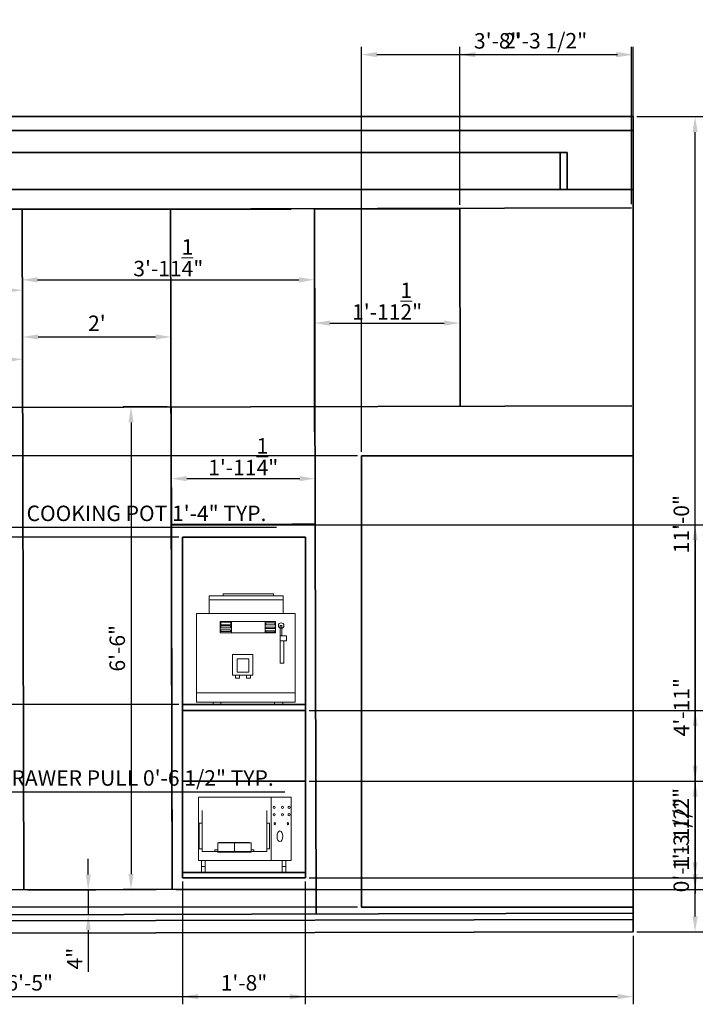
# Model space of a CAD drawing. Units: inches. Extents: x 1464 to 1689, y 996 to 1156.
# Tile 2 of 2: x 1578 to 1689, y 997 to 1156. Entities that reach past the tile are written whole.
import ezdxf

# ---------------------------------------------------------------- set-up
doc = ezdxf.new("R2010")
doc.units = ezdxf.units.IN
for name, color, linetype, lineweight in [('A-ANNO-DIMS', 2, 'Continuous', 18), ('A-ELEV', 7, 'Continuous', 35), ('A-EQPM', 9, 'Continuous', 18)]:
    doc.layers.add(name, color=color, linetype=linetype, lineweight=lineweight)
doc.styles.get("Standard").update_dxf_attribs({"font": 'arial.ttf'})
doc.dimstyles.new('ISO-25', dxfattribs={"dimtxt": 2.5, "dimasz": 2.5, "dimexe": 1.25, "dimexo": 0.625, "dimtad": 1, "dimdec": 4, "dimlunit": 4, "dimtxsty": 'Standard', "dimcen": 2.5, "dimadec": 0, "dimazin": 0, "dimtfac": 1, "dimtdec": 4, "dimtmove": 0, "dimatfit": 3, "dimfxl": 1, "dimarcsym": 0})

# ---------------------------------------------------------------- blocks, each defined once
blk = doc.blocks.new('*D3')
at = {"layer": 'A-ANNO-DIMS', "color": 0, "lineweight": -2, "transparency": 16777216}
for p, q in [((1534.7, 1124.64), (1534.7, 1110.94)), ((1578.2, 1124.64), (1578.2, 1110.94)), ((1575.7, 1112.19), (1537.2, 1112.19))]:
    blk.add_line(p, q, dxfattribs=at)
at = {"layer": 'A-ANNO-DIMS', "color": 0, "transparency": 16777216}
for points in [[(1537.2, 1112.6), (1537.2, 1111.77), (1534.7, 1112.19)], [(1575.7, 1112.6), (1575.7, 1111.77), (1578.2, 1112.19)]]:
    blk.add_solid(points, dxfattribs=at)
at = {"layer": 'Defpoints', "color": 0, "transparency": 16777216}
for p in [(1534.7, 1125.27), (1578.2, 1125.27), (1534.7, 1112.19)]:
    blk.add_point(p, dxfattribs=at)
at = {"layer": 'A-ANNO-DIMS', "color": 0, "transparency": 16777216, "insert": (1556.45, 1115.76), "char_height": 2.5, "attachment_point": 5}
blk.add_mtext('3\'-7{\\H1x;\\S1/2;}"', dxfattribs=at)
blk = doc.blocks.new('*D5')
at = {"layer": 'A-ANNO-DIMS', "color": 0, "lineweight": -2, "transparency": 16777216}
for p, q in [((1601.65, 1093.32), (1594.55, 1093.32)), ((1595.8, 1090.82), (1595.8, 1017.82)), ((1601.83, 1015.32), (1594.55, 1015.32))]:
    blk.add_line(p, q, dxfattribs=at)
at = {"layer": 'A-ANNO-DIMS', "color": 0, "transparency": 16777216}
for points in [[(1595.39, 1090.82), (1596.22, 1090.82), (1595.8, 1093.32)], [(1595.39, 1017.82), (1596.22, 1017.82), (1595.8, 1015.32)]]:
    blk.add_solid(points, dxfattribs=at)
at = {"layer": 'Defpoints', "color": 0, "transparency": 16777216}
for p in [(1602.28, 1093.32), (1595.8, 1015.32), (1602.45, 1015.32)]:
    blk.add_point(p, dxfattribs=at)
at = {"layer": 'A-ANNO-DIMS', "color": 0, "transparency": 16777216, "insert": (1593.9, 1054.32), "char_height": 2.5, "attachment_point": 5, "rotation": 90}
blk.add_mtext('6\'-6"', dxfattribs=at)
blk = doc.blocks.new('*D7')
at = {"layer": 'A-ANNO-DIMS', "color": 0, "lineweight": -2, "transparency": 16777216}
for p, q in [((1602.32, 1074.89), (1602.32, 1082.98)), ((1625.57, 1074.89), (1625.57, 1082.98)), ((1623.07, 1081.73), (1604.82, 1081.73))]:
    blk.add_line(p, q, dxfattribs=at)
at = {"layer": 'A-ANNO-DIMS', "color": 0, "transparency": 16777216}
for points in [[(1604.82, 1082.15), (1604.82, 1081.32), (1602.32, 1081.73)], [(1623.07, 1082.15), (1623.07, 1081.32), (1625.57, 1081.73)]]:
    blk.add_solid(points, dxfattribs=at)
at = {"layer": 'Defpoints', "color": 0, "transparency": 16777216}
for p in [(1602.32, 1081.73), (1602.32, 1074.27), (1625.57, 1074.27)]:
    blk.add_point(p, dxfattribs=at)
at = {"layer": 'A-ANNO-DIMS', "color": 0, "transparency": 16777216, "insert": (1613.94, 1085.28), "char_height": 2.5, "attachment_point": 5}
blk.add_mtext('1\'-11{\\H1x;\\S1/4;}"', dxfattribs=at)
blk = doc.blocks.new('*D8')
at = {"layer": 'A-ANNO-DIMS', "color": 0, "lineweight": -2, "transparency": 16777216}
for p, q in [((1625.45, 1124.75), (1625.45, 1105.63)), ((1648.95, 1124.75), (1648.95, 1105.63)), ((1627.95, 1106.88), (1646.45, 1106.88))]:
    blk.add_line(p, q, dxfattribs=at)
at = {"layer": 'A-ANNO-DIMS', "color": 0, "transparency": 16777216}
for points in [[(1627.95, 1107.29), (1627.95, 1106.46), (1625.45, 1106.88)], [(1646.45, 1107.29), (1646.45, 1106.46), (1648.95, 1106.88)]]:
    blk.add_solid(points, dxfattribs=at)
at = {"layer": 'Defpoints', "color": 0, "transparency": 16777216}
for p in [(1625.45, 1125.37), (1648.95, 1125.37), (1648.95, 1106.88)]:
    blk.add_point(p, dxfattribs=at)
at = {"layer": 'A-ANNO-DIMS', "color": 0, "transparency": 16777216, "insert": (1637.2, 1110.43), "char_height": 2.5, "attachment_point": 5}
blk.add_mtext('1\'-11{\\H1x;\\S1/2;}"', dxfattribs=at)
blk = doc.blocks.new('*D9')
at = {"layer": 'A-ANNO-DIMS', "color": 0, "lineweight": -2, "transparency": 16777216}
for p, q in [((1554.53, 1093.84), (1554.53, 1102.26)), ((1578.28, 1093.89), (1578.28, 1102.26)), ((1557.03, 1101.01), (1575.78, 1101.01))]:
    blk.add_line(p, q, dxfattribs=at)
at = {"layer": 'A-ANNO-DIMS', "color": 0, "transparency": 16777216}
for points in [[(1557.03, 1101.43), (1557.03, 1100.6), (1554.53, 1101.01)], [(1575.78, 1101.43), (1575.78, 1100.6), (1578.28, 1101.01)]]:
    blk.add_solid(points, dxfattribs=at)
at = {"layer": 'Defpoints', "color": 0, "transparency": 16777216}
for p in [(1578.28, 1101.01), (1554.53, 1093.21), (1578.28, 1093.27)]:
    blk.add_point(p, dxfattribs=at)
at = {"layer": 'A-ANNO-DIMS', "color": 0, "transparency": 16777216, "insert": (1566.4, 1104.58), "char_height": 2.5, "attachment_point": 5}
blk.add_mtext('1\'-11{\\H1x;\\S3/4;}"', dxfattribs=at)
blk = doc.blocks.new('*D10')
at = {"layer": 'A-ANNO-DIMS', "color": 0, "lineweight": -2, "transparency": 16777216}
for p, q in [((1578.28, 1093.89), (1578.28, 1105.89)), ((1580.78, 1104.64), (1599.78, 1104.64)), ((1602.28, 1093.95), (1602.28, 1105.89))]:
    blk.add_line(p, q, dxfattribs=at)
at = {"layer": 'A-ANNO-DIMS', "color": 0, "transparency": 16777216}
for points in [[(1580.78, 1105.06), (1580.78, 1104.23), (1578.28, 1104.64)], [(1599.78, 1105.06), (1599.78, 1104.23), (1602.28, 1104.64)]]:
    blk.add_solid(points, dxfattribs=at)
at = {"layer": 'Defpoints', "color": 0, "transparency": 16777216}
for p in [(1602.28, 1104.64), (1578.28, 1093.27), (1602.28, 1093.32)]:
    blk.add_point(p, dxfattribs=at)
at = {"layer": 'A-ANNO-DIMS', "color": 0, "transparency": 16777216, "insert": (1590.28, 1106.52), "char_height": 2.5, "attachment_point": 5}
blk.add_mtext("2'", dxfattribs=at)
blk = doc.blocks.new('*D11')
at = {"layer": 'A-ANNO-DIMS', "color": 0, "lineweight": -2, "transparency": 16777216}
for p, q in [((1578.2, 1124.64), (1578.2, 1112.62)), ((1625.45, 1124.64), (1625.45, 1112.62)), ((1580.7, 1113.87), (1622.95, 1113.87))]:
    blk.add_line(p, q, dxfattribs=at)
at = {"layer": 'A-ANNO-DIMS', "color": 0, "transparency": 16777216}
for points in [[(1580.7, 1114.28), (1580.7, 1113.45), (1578.2, 1113.87)], [(1622.95, 1114.28), (1622.95, 1113.45), (1625.45, 1113.87)]]:
    blk.add_solid(points, dxfattribs=at)
at = {"layer": 'Defpoints', "color": 0, "transparency": 16777216}
for p in [(1578.2, 1125.27), (1625.45, 1125.27), (1625.45, 1113.87)]:
    blk.add_point(p, dxfattribs=at)
at = {"layer": 'A-ANNO-DIMS', "color": 0, "transparency": 16777216, "insert": (1601.83, 1117.44), "char_height": 2.5, "attachment_point": 5}
blk.add_mtext('3\'-11{\\H1x;\\S1/4;}"', dxfattribs=at)
blk = doc.blocks.new('*D12')
at = {"layer": 'A-ANNO-DIMS', "color": 0, "lineweight": -2, "transparency": 16777216}
for p, q in [((1588.88, 1017.77), (1588.88, 1020.27)), ((1579.08, 1015.27), (1590.13, 1015.27)), ((1588.88, 1015.27), (1588.88, 1011.27)), ((1579.09, 1011.27), (1590.13, 1011.27)), ((1588.88, 1008.77), (1588.88, 1002.04))]:
    blk.add_line(p, q, dxfattribs=at)
at = {"layer": 'A-ANNO-DIMS', "color": 0, "transparency": 16777216}
for points in [[(1588.47, 1017.77), (1589.3, 1017.77), (1588.88, 1015.27)], [(1588.47, 1008.77), (1589.3, 1008.77), (1588.88, 1011.27)]]:
    blk.add_solid(points, dxfattribs=at)
at = {"layer": 'Defpoints', "color": 0, "transparency": 16777216}
for p in [(1578.45, 1015.27), (1578.46, 1011.27), (1588.88, 1011.27)]:
    blk.add_point(p, dxfattribs=at)
at = {"layer": 'A-ANNO-DIMS', "color": 0, "transparency": 16777216, "insert": (1587.01, 1004.15), "char_height": 2.5, "attachment_point": 5, "rotation": 90}
blk.add_mtext('4"', dxfattribs=at)
blk = doc.blocks.new('*D16')
at = {"layer": 'A-ANNO-DIMS', "color": 0, "lineweight": -2, "transparency": 16777216}
for p, q in [((1563.08, 1030.73), (1563.08, 1032.37)), ((1569.81, 1030.73), (1569.81, 1032.37)), ((1565.58, 1031.12), (1567.31, 1031.12)), ((1569.81, 1031.12), (1620.69, 1031.12))]:
    blk.add_line(p, q, dxfattribs=at)
at = {"layer": 'A-ANNO-DIMS', "color": 0, "transparency": 16777216}
for points in [[(1565.58, 1031.53), (1565.58, 1030.7), (1563.08, 1031.12)], [(1567.31, 1031.53), (1567.31, 1030.7), (1569.81, 1031.12)]]:
    blk.add_solid(points, dxfattribs=at)
at = {"layer": 'Defpoints', "color": 0, "transparency": 16777216}
for p in [(1563.08, 1030.11), (1569.81, 1031.12), (1569.81, 1030.11)]:
    blk.add_point(p, dxfattribs=at)
at = {"layer": 'A-ANNO-DIMS', "color": 0, "transparency": 16777216, "insert": (1596.5, 1033.03), "char_height": 2.5, "attachment_point": 5}
blk.add_mtext('DRAWER PULL 0\'-6 1/2" TYP.', dxfattribs=at)
blk = doc.blocks.new('*D18')
at = {"layer": 'A-ANNO-DIMS', "color": 0, "lineweight": -2, "transparency": 16777216}
for p, q in [((1558.97, 1072.14), (1558.97, 1075.13)), ((1574.77, 1072.14), (1574.77, 1075.13)), ((1561.47, 1073.88), (1572.27, 1073.88)), ((1574.77, 1073.88), (1619.34, 1073.88))]:
    blk.add_line(p, q, dxfattribs=at)
at = {"layer": 'A-ANNO-DIMS', "color": 0, "transparency": 16777216}
for points in [[(1561.47, 1074.3), (1561.47, 1073.46), (1558.97, 1073.88)], [(1572.27, 1074.3), (1572.27, 1073.46), (1574.77, 1073.88)]]:
    blk.add_solid(points, dxfattribs=at)
at = {"layer": 'Defpoints', "color": 0, "transparency": 16777216}
for p in [(1574.77, 1073.88), (1558.97, 1071.51), (1574.77, 1071.51)]:
    blk.add_point(p, dxfattribs=at)
at = {"layer": 'A-ANNO-DIMS', "color": 0, "transparency": 16777216, "insert": (1598.3, 1075.8), "char_height": 2.5, "attachment_point": 5}
blk.add_mtext('COOKING POT 1\'-4" TYP.', dxfattribs=at)
blk = doc.blocks.new('*D20')
at = {"layer": 'A-ANNO-DIMS', "color": 0, "lineweight": -2, "transparency": 16777216}
for p, q in [((1479.97, 1007.42), (1479.97, 996.77)), ((1676.97, 1007.86), (1676.97, 996.77)), ((1482.47, 998.02), (1674.47, 998.02))]:
    blk.add_line(p, q, dxfattribs=at)
at = {"layer": 'A-ANNO-DIMS', "color": 0, "transparency": 16777216}
for points in [[(1482.47, 998.44), (1482.47, 997.6), (1479.97, 998.02)], [(1674.47, 998.44), (1674.47, 997.6), (1676.97, 998.02)]]:
    blk.add_solid(points, dxfattribs=at)
at = {"layer": 'Defpoints', "color": 0, "transparency": 16777216}
for p in [(1479.97, 1008.05), (1676.97, 1008.49), (1676.97, 998.02)]:
    blk.add_point(p, dxfattribs=at)
at = {"layer": 'A-ANNO-DIMS', "color": 0, "transparency": 16777216, "insert": (1578.47, 999.92), "char_height": 2.5, "attachment_point": 5}
blk.add_mtext('16\'-5"', dxfattribs=at)
blk = doc.blocks.new('*D21')
at = {"layer": 'A-ANNO-DIMS', "color": 0, "lineweight": -2, "transparency": 16777216}
for p, q in [((1677.59, 1140.25), (1688.24, 1140.25)), ((1686.99, 1010.99), (1686.99, 1137.75)), ((1677.59, 1008.49), (1688.24, 1008.49))]:
    blk.add_line(p, q, dxfattribs=at)
at = {"layer": 'A-ANNO-DIMS', "color": 0, "transparency": 16777216}
for points in [[(1686.58, 1137.75), (1687.41, 1137.75), (1686.99, 1140.25)], [(1686.58, 1010.99), (1687.41, 1010.99), (1686.99, 1008.49)]]:
    blk.add_solid(points, dxfattribs=at)
at = {"layer": 'Defpoints', "color": 0, "transparency": 16777216}
for p in [(1676.97, 1140.25), (1686.99, 1140.25), (1676.97, 1008.49)]:
    blk.add_point(p, dxfattribs=at)
at = {"layer": 'A-ANNO-DIMS', "color": 0, "transparency": 16777216, "insert": (1685.09, 1074.37), "char_height": 2.5, "attachment_point": 5, "rotation": 90}
blk.add_mtext('11\'-0"', dxfattribs=at)
blk = doc.blocks.new('*D26')
at = {"layer": 'A-ANNO-DIMS', "color": 0, "lineweight": -2, "transparency": 16777216}
for p, q in [((1648.95, 1126), (1648.95, 1151.52)), ((1676.7, 1126.11), (1676.7, 1151.52)), ((1651.45, 1150.27), (1674.2, 1150.27))]:
    blk.add_line(p, q, dxfattribs=at)
at = {"layer": 'A-ANNO-DIMS', "color": 0, "transparency": 16777216}
for points in [[(1651.45, 1150.69), (1651.45, 1149.86), (1648.95, 1150.27)], [(1674.2, 1150.69), (1674.2, 1149.86), (1676.7, 1150.27)]]:
    blk.add_solid(points, dxfattribs=at)
at = {"layer": 'Defpoints', "color": 0, "transparency": 16777216}
for p in [(1676.7, 1150.27), (1648.95, 1125.37), (1676.7, 1125.49)]:
    blk.add_point(p, dxfattribs=at)
at = {"layer": 'A-ANNO-DIMS', "color": 0, "transparency": 16777216, "insert": (1662.83, 1152.19), "char_height": 2.5, "attachment_point": 5}
blk.add_mtext('2\'-3 1/2"', dxfattribs=at)
blk = doc.blocks.new('*D27')
at = {"layer": 'A-ANNO-DIMS', "color": 0, "lineweight": -2, "transparency": 16777216}
for p, q in [((1632.43, 1085.44), (1468.43, 1085.44)), ((1469.68, 1014.98), (1469.68, 1082.94)), ((1632.43, 1012.48), (1468.43, 1012.48))]:
    blk.add_line(p, q, dxfattribs=at)
at = {"layer": 'A-ANNO-DIMS', "color": 0, "transparency": 16777216}
for points in [[(1469.26, 1082.94), (1470.1, 1082.94), (1469.68, 1085.44)], [(1469.26, 1014.98), (1470.1, 1014.98), (1469.68, 1012.48)]]:
    blk.add_solid(points, dxfattribs=at)
at = {"layer": 'Defpoints', "color": 0, "transparency": 16777216}
for p in [(1469.68, 1085.44), (1633.05, 1085.44), (1633.05, 1012.48)]:
    blk.add_point(p, dxfattribs=at)
at = {"layer": 'A-ANNO-DIMS', "color": 0, "transparency": 16777216, "insert": (1467.78, 1048.96), "char_height": 2.5, "attachment_point": 5, "rotation": 90}
blk.add_mtext('6\'-1"', dxfattribs=at)
blk = doc.blocks.new('*D28')
at = {"layer": 'A-ANNO-DIMS', "color": 0, "lineweight": -2, "transparency": 16777216}
for p, q in [((1633.05, 1086.06), (1633.05, 1151.52)), ((1676.97, 1086.06), (1676.97, 1151.52)), ((1635.55, 1150.27), (1674.47, 1150.27))]:
    blk.add_line(p, q, dxfattribs=at)
at = {"layer": 'A-ANNO-DIMS', "color": 0, "transparency": 16777216}
for points in [[(1635.55, 1150.69), (1635.55, 1149.86), (1633.05, 1150.27)], [(1674.47, 1150.69), (1674.47, 1149.86), (1676.97, 1150.27)]]:
    blk.add_solid(points, dxfattribs=at)
at = {"layer": 'Defpoints', "color": 0, "transparency": 16777216}
for p in [(1676.97, 1150.27), (1633.05, 1085.44), (1676.97, 1085.44)]:
    blk.add_point(p, dxfattribs=at)
at = {"layer": 'A-ANNO-DIMS', "color": 0, "transparency": 16777216, "insert": (1655.01, 1152.17), "char_height": 2.5, "attachment_point": 5}
blk.add_mtext('3\'-8"', dxfattribs=at)
blk = doc.blocks.new('*D41')
at = {"layer": 'A-ANNO-DIMS', "color": 0, "lineweight": -2, "transparency": 16777216}
for p, q in [((1602.94, 1074.27), (1688.24, 1074.27)), ((1686.99, 1071.77), (1686.99, 1017.82)), ((1603.08, 1015.32), (1688.24, 1015.32))]:
    blk.add_line(p, q, dxfattribs=at)
at = {"layer": 'A-ANNO-DIMS', "color": 0, "transparency": 16777216}
for points in [[(1686.58, 1071.77), (1687.41, 1071.77), (1686.99, 1074.27)], [(1686.58, 1017.82), (1687.41, 1017.82), (1686.99, 1015.32)]]:
    blk.add_solid(points, dxfattribs=at)
at = {"layer": 'Defpoints', "color": 0, "transparency": 16777216}
for p in [(1602.32, 1074.27), (1602.45, 1015.32), (1686.99, 1015.32)]:
    blk.add_point(p, dxfattribs=at)
at = {"layer": 'A-ANNO-DIMS', "color": 0, "transparency": 16777216, "insert": (1685.11, 1044.79), "char_height": 2.5, "attachment_point": 5, "rotation": 90}
blk.add_mtext('4\'-11"', dxfattribs=at)
blk = doc.blocks.new('*D42')
at = {"layer": 'A-ANNO-DIMS', "color": 0, "lineweight": -2, "transparency": 16777216}
for p, q in [((1603.51, 1072.27), (1468.43, 1072.27)), ((1469.68, 1069.77), (1469.68, 1047.75)), ((1603.51, 1045.25), (1468.43, 1045.25))]:
    blk.add_line(p, q, dxfattribs=at)
at = {"layer": 'A-ANNO-DIMS', "color": 0, "transparency": 16777216}
for points in [[(1469.26, 1069.77), (1470.1, 1069.77), (1469.68, 1072.27)], [(1469.26, 1047.75), (1470.1, 1047.75), (1469.68, 1045.25)]]:
    blk.add_solid(points, dxfattribs=at)
at = {"layer": 'Defpoints', "color": 0, "transparency": 16777216}
for p in [(1604.13, 1072.27), (1469.68, 1045.25), (1604.13, 1045.25)]:
    blk.add_point(p, dxfattribs=at)
at = {"layer": 'A-ANNO-DIMS', "color": 0, "transparency": 16777216, "insert": (1467.78, 1058.76), "char_height": 2.5, "attachment_point": 5, "rotation": 90}
blk.add_mtext('2\'-3"', dxfattribs=at)
blk = doc.blocks.new('*D43')
at = {"layer": 'A-ANNO-DIMS', "color": 0, "lineweight": -2, "transparency": 16777216}
for p, q in [((1624.61, 1044.25), (1688.24, 1044.25)), ((1686.99, 1041.75), (1686.99, 1035.35)), ((1624.61, 1032.85), (1688.24, 1032.85)), ((1686.99, 1032.85), (1686.99, 1014.69))]:
    blk.add_line(p, q, dxfattribs=at)
at = {"layer": 'A-ANNO-DIMS', "color": 0, "transparency": 16777216}
for points in [[(1686.58, 1041.75), (1687.41, 1041.75), (1686.99, 1044.25)], [(1686.58, 1035.35), (1687.41, 1035.35), (1686.99, 1032.85)]]:
    blk.add_solid(points, dxfattribs=at)
at = {"layer": 'Defpoints', "color": 0, "transparency": 16777216}
for p in [(1623.98, 1044.25), (1623.98, 1032.85), (1686.99, 1032.85)]:
    blk.add_point(p, dxfattribs=at)
at = {"layer": 'A-ANNO-DIMS', "color": 0, "transparency": 16777216, "insert": (1685.07, 1022.52), "char_height": 2.5, "attachment_point": 5, "rotation": 90}
blk.add_mtext('0\'-11 1/2"', dxfattribs=at)
blk = doc.blocks.new('*D44')
at = {"layer": 'A-ANNO-DIMS', "color": 0, "lineweight": -2, "transparency": 16777216}
for p, q in [((1624.61, 1032.85), (1688.24, 1032.85)), ((1686.99, 1030.35), (1686.99, 1019.73)), ((1624.61, 1017.23), (1688.24, 1017.23))]:
    blk.add_line(p, q, dxfattribs=at)
at = {"layer": 'A-ANNO-DIMS', "color": 0, "transparency": 16777216}
for points in [[(1686.58, 1030.35), (1687.41, 1030.35), (1686.99, 1032.85)], [(1686.58, 1019.73), (1687.41, 1019.73), (1686.99, 1017.23)]]:
    blk.add_solid(points, dxfattribs=at)
at = {"layer": 'Defpoints', "color": 0, "transparency": 16777216}
for p in [(1623.98, 1032.85), (1623.98, 1017.23), (1686.99, 1017.23)]:
    blk.add_point(p, dxfattribs=at)
at = {"layer": 'A-ANNO-DIMS', "color": 0, "transparency": 16777216, "insert": (1685.07, 1025.04), "char_height": 2.5, "attachment_point": 5, "rotation": 90}
blk.add_mtext('1\'-3 1/2"', dxfattribs=at)
blk = doc.blocks.new('*D45')
at = {"layer": 'A-ANNO-DIMS', "color": 0, "lineweight": -2, "transparency": 16777216}
for p, q in [((1604.13, 1016.61), (1604.13, 996.77)), ((1623.98, 1016.61), (1623.98, 996.77)), ((1606.63, 998.02), (1621.48, 998.02))]:
    blk.add_line(p, q, dxfattribs=at)
at = {"layer": 'A-ANNO-DIMS', "color": 0, "transparency": 16777216}
for points in [[(1606.63, 998.44), (1606.63, 997.6), (1604.13, 998.02)], [(1621.48, 998.44), (1621.48, 997.6), (1623.98, 998.02)]]:
    blk.add_solid(points, dxfattribs=at)
at = {"layer": 'Defpoints', "color": 0, "transparency": 16777216}
for p in [(1604.13, 1017.23), (1623.98, 1017.23), (1623.98, 998.02)]:
    blk.add_point(p, dxfattribs=at)
at = {"layer": 'A-ANNO-DIMS', "color": 0, "transparency": 16777216, "insert": (1614.06, 999.92), "char_height": 2.5, "attachment_point": 5}
blk.add_mtext('1\'-8"', dxfattribs=at)

msp = doc.modelspace()

# ---------------------------------------------------------------- linework, layer by layer
at = {"layer": 'A-ELEV'}
for p, q in [((1479.96715, 1140.24723), (1676.96715, 1140.24723)), ((1676.96715, 1140.24723), (1676.96715, 1128.48751)), ((1676.96715, 1140.24723), (1676.96715, 1138.01467)), ((1676.96715, 1138.01467), (1479.96715, 1138.01467)), ((1501.63185, 1134.453), (1666.33231, 1134.453)), ((1665.1789, 1134.453), (1665.1789, 1128.48751)), ((1666.33231, 1134.453), (1666.33231, 1128.48751)), ((1676.96715, 1128.48751), (1479.96715, 1128.48751)), ((1676.96715, 1008.48751), (1676.96715, 1128.48751)), ((1479.70522, 1125.04535), (1676.70473, 1125.48722)), ((1578.20497, 1125.26628), (1534.70497, 1125.26628)), ((1578.20497, 1125.26628), (1554.45497, 1125.26628)), ((1578.4517, 1015.26656), (1578.20497, 1125.26628)), ((1578.20497, 1125.26628), (1602.20497, 1125.26628)), ((1578.20497, 1125.26628), (1621.70497, 1125.26628)), ((1602.20497, 1125.26628), (1602.45158, 1015.32039)), ((1625.56937, 1074.26641), (1625.45474, 1125.37226)), ((1625.45474, 1125.37226), (1625.45474, 1089.37226)), ((1625.45474, 1125.37226), (1648.95474, 1125.37226)), ((1648.95474, 1125.37226), (1649.02639, 1093.42505)), ((1479.777, 1093.04543), (1676.7765, 1093.4873)), ((1602.27663, 1093.3202), (1602.45158, 1015.32039)), ((1602.31924, 1074.32024), (1625.56913, 1074.37239)), ((1602.31937, 1074.26641), (1625.56937, 1074.26641)), ((1621.81915, 1074.36398), (1625.56915, 1074.36398)), ((1625.56937, 1074.26641), (1625.71043, 1011.37255)), ((1623.98434, 1072.27429), (1604.13436, 1072.27429)), ((1604.13436, 1072.27429), (1604.13436, 1017.23218)), ((1623.98434, 1017.23218), (1623.98434, 1072.27429)), ((1604.13436, 1045.25324), (1623.98434, 1045.25324)), ((1604.13436, 1044.25324), (1623.98434, 1044.25324)), ((1604.13436, 1017.23218), (1623.98434, 1017.23218)), ((1479.95195, 1015.04563), (1625.70146, 1015.37254)), ((1479.96092, 1011.04564), (1676.96042, 1011.4875)), ((1479.96316, 1010.04564), (1676.96267, 1010.48751)), ((1479.96765, 1008.04565), (1676.96715, 1008.48751))]:
    msp.add_line(p, q, dxfattribs=at)
for points in [[(1633.05067, 1085.4387), (1676.96715, 1085.4387), (1676.96715, 1012.47552), (1633.05067, 1012.47552)], [(1604.13436, 1032.85015), (1623.98434, 1032.85015), (1623.98434, 1018.06918), (1604.13436, 1018.06918)]]:
    msp.add_lwpolyline(points, close=True, dxfattribs=at)
at = {"layer": 'A-EQPM'}
for p, q in [((1610.71858, 1062.7729), (1610.71858, 1063.14033)), ((1610.71858, 1063.14033), (1618.82353, 1063.14033)), ((1618.82353, 1063.14033), (1618.82353, 1062.7729)), ((1608.45893, 1059.93647), (1608.45893, 1062.7729)), ((1608.45893, 1062.7729), (1620.40305, 1062.7729)), ((1608.45893, 1062.14355), (1620.40305, 1062.14355)), ((1620.40305, 1062.7729), (1620.40305, 1059.93647)), ((1606.37558, 1059.93647), (1622.33888, 1059.93647)), ((1606.37558, 1045.63071), (1606.37558, 1059.93647)), ((1622.33888, 1059.93647), (1622.33888, 1045.63071)), ((1611.91917, 1058.53051), (1610.34375, 1058.53051)), ((1610.34375, 1058.53051), (1610.34375, 1058.10265)), ((1610.34375, 1058.49822), (1610.34375, 1058.10265)), ((1611.91917, 1058.10265), (1611.91917, 1058.53051)), ((1610.34375, 1058.10265), (1611.91917, 1058.10265)), ((1606.37558, 1047.11691), (1622.33888, 1047.11691)), ((1622.33888, 1045.63071), (1606.37558, 1045.63071)), ((1609.06938, 1045.63071), (1609.06938, 1045.25324)), ((1610.31062, 1045.25324), (1610.31062, 1045.63071)), ((1619.0177, 1045.25324), (1619.0177, 1045.63071)), ((1619.0177, 1045.63071), (1620.35884, 1045.63071)), ((1620.35884, 1045.63071), (1620.35884, 1045.25324)), ((1609.06938, 1045.25324), (1610.31062, 1045.25324)), ((1610.38565, 1032.85015), (1610.49442, 1032.85015)), ((1618.44654, 1030.24174), (1618.44654, 1020.02549)), ((1607.29188, 1028.08153), (1607.29188, 1021.47019)), ((1617.73098, 1021.47019), (1617.73098, 1028.08153)), ((1607.29188, 1026.05225), (1606.83007, 1026.05225)), ((1606.83007, 1026.05225), (1606.83007, 1021.90644)), ((1617.73098, 1026.05225), (1618.19279, 1026.05225)), ((1618.19279, 1026.05225), (1618.19279, 1021.90644)), ((1606.83007, 1021.90644), (1607.29188, 1021.90644)), ((1609.36815, 1021.74854), (1609.81141, 1021.74854)), ((1609.36815, 1021.74854), (1609.36815, 1021.47019)), ((1612.51143, 1022.86546), (1609.81141, 1022.86546)), ((1609.81141, 1022.86546), (1609.81141, 1021.47019)), ((1609.97471, 1022.86546), (1609.97471, 1022.94566)), ((1609.97471, 1022.94566), (1614.96912, 1022.94566)), ((1612.51143, 1021.47019), (1612.51143, 1022.86546)), ((1612.51143, 1022.86546), (1615.21145, 1022.86546)), ((1612.51143, 1021.47019), (1612.51143, 1022.86546)), ((1614.96912, 1022.94566), (1614.96912, 1022.86546)), ((1615.21145, 1022.86546), (1615.21145, 1021.47019)), ((1615.65471, 1021.74854), (1615.21145, 1021.74854)), ((1615.65471, 1021.47019), (1615.65471, 1021.74854)), ((1618.19279, 1021.90644), (1617.73098, 1021.90644)), ((1607.29188, 1021.47019), (1617.73098, 1021.47019)), ((1609.81141, 1021.47019), (1609.36815, 1021.47019)), ((1609.81141, 1021.47019), (1609.80385, 1021.47019)), ((1609.80385, 1021.47019), (1609.80385, 1021.33524)), ((1609.80385, 1021.33524), (1612.51143, 1021.33524)), ((1612.51143, 1021.33524), (1612.51143, 1021.47019)), ((1612.51143, 1021.33524), (1612.51143, 1021.47019)), ((1615.21901, 1021.33524), (1612.51143, 1021.33524)), ((1615.21145, 1021.47019), (1615.65471, 1021.47019)), ((1615.21145, 1021.47019), (1615.21901, 1021.47019)), ((1615.21901, 1021.47019), (1615.21901, 1021.33524)), ((1607.18652, 1020.02549), (1607.18652, 1018.06918)), ((1607.18652, 1019.04734), (1607.76735, 1019.04734)), ((1607.76735, 1020.02549), (1607.76735, 1018.06918)), ((1620.25516, 1020.02549), (1620.25516, 1018.06918)), ((1620.25516, 1019.04734), (1620.836, 1019.04734)), ((1620.836, 1020.02549), (1620.836, 1018.06918))]:
    msp.add_line(p, q, dxfattribs=at)
for points in [[(1612.0701, 1058.63869), (1610.1991, 1058.63869), (1610.1991, 1056.83508), (1612.0701, 1056.83508)], [(1612.0701, 1058.63869), (1617.47224, 1058.63869), (1617.47224, 1056.81455), (1612.0701, 1056.81455)], [(1617.47224, 1058.63869), (1619.13643, 1058.63869), (1619.13643, 1056.79402), (1617.47224, 1056.79402)], [(1617.59064, 1058.44171), (1619.0287, 1058.44171), (1619.0287, 1058.0865), (1617.59064, 1058.0865)], [(1610.34375, 1057.92505), (1611.90301, 1057.92505), (1611.90301, 1057.63442), (1610.34375, 1057.63442)], [(1610.34375, 1057.28728), (1611.90301, 1057.28728), (1611.90301, 1057.0128), (1610.34375, 1057.0128)], [(1617.59064, 1057.75551), (1619.0287, 1057.75551), (1619.0287, 1057.48911), (1617.59064, 1057.48911)], [(1617.59064, 1057.14197), (1619.0287, 1057.14197), (1619.0287, 1056.93207), (1617.59064, 1056.93207)], [(1619.93772, 1056.35439), (1620.1987, 1056.35439), (1620.1987, 1057.99058), (1619.93772, 1057.99058)], [(1619.93772, 1055.54252), (1620.93301, 1055.54252), (1620.93301, 1056.35439), (1619.93772, 1056.35439)], [(1619.93772, 1055.54252), (1620.50646, 1055.54252), (1620.50646, 1051.90942), (1619.93772, 1051.90942)], [(1612.22945, 1053.32793), (1615.47307, 1053.32793), (1615.47307, 1049.9905), (1612.22945, 1049.9905)], [(1612.93598, 1052.58984), (1614.86288, 1052.58984), (1614.86288, 1050.43977), (1612.93598, 1050.43977)], [(1612.71119, 1049.9905), (1613.32137, 1049.9905), (1613.32137, 1049.50914), (1612.71119, 1049.50914)], [(1614.44539, 1049.9905), (1615.09643, 1049.9905), (1615.09643, 1049.50914), (1614.44539, 1049.50914)], [(1606.68762, 1030.24174), (1621.69728, 1030.24174), (1621.69728, 1020.02549), (1606.68762, 1020.02549)]]:
    msp.add_lwpolyline(points, close=True, dxfattribs=at)
for centre, radius in [((1620.06821, 1057.99058), 0.44546), ((1618.94761, 1028.59418), 0.18152), ((1620.29264, 1028.59418), 0.18152), ((1621.361, 1028.59418), 0.18152), ((1618.94761, 1027.41556), 0.18152), ((1620.29264, 1027.41556), 0.18152), ((1621.361, 1027.41556), 0.18152)]:
    msp.add_circle(centre, radius, dxfattribs=at)
for centre, major_axis, ratio in [((1619.03477, 1025.98122), (0.00044, 0.18039), 0.612589674), ((1621.16588, 1025.98122), (0.00044, 0.18039), 0.612589674), ((1619.87554, 1023.92983), (0, 0.86063), 0.533330578)]:
    msp.add_ellipse(centre, major_axis=major_axis, ratio=ratio, dxfattribs=at)

# ---------------------------------------------------------------- dimensions: what is measured, and where the dimension line sits
at = {"layer": 'A-ANNO-DIMS'}
for base, p1, p2, override, picture, middle in [((1676.70473, 1150.27223), (1648.95474, 1125.37226), (1676.70473, 1125.48722), {"dimdec": 1, "dimlfac": 1, "dimrnd": 0, "dimzin": 1, "dimdsep": 46, "dimlunit": 4, "dimfrac": 2}, '*D26', (1662.82973, 1152.19071)), ((1676.96715, 1150.27223), (1633.05067, 1085.4387), (1676.96715, 1085.4387), {"dimdec": 1, "dimlfac": 1, "dimrnd": 0, "dimzin": 1, "dimdsep": 46, "dimlunit": 4, "dimfrac": 2}, '*D28', (1655.00891, 1152.17451)), ((1534.70497, 1112.18674), (1578.20497, 1125.26628), (1534.70497, 1125.26628), {"dimclrd": 0, "dimclre": 0, "dimclrt": 0}, '*D3', (1556.45497, 1115.76081)), ((1625.45474, 1113.86824), (1578.20497, 1125.26628), (1625.45474, 1125.26628), {"dimclrd": 0, "dimclre": 0, "dimclrt": 0}, '*D11', (1601.82985, 1117.43719)), ((1648.95474, 1106.87813), (1625.45474, 1125.37226), (1648.95474, 1125.37226), {"dimclrd": 0, "dimclre": 0, "dimclrt": 0}, '*D8', (1637.20474, 1110.43003)), ((1602.27663, 1104.64292), (1578.27675, 1093.26636), (1602.27663, 1093.3202), {"dimclrd": 0, "dimclre": 0, "dimclrt": 0}, '*D10', (1590.27669, 1106.52303)), ((1578.27675, 1101.014), (1554.52687, 1093.21309), (1578.27675, 1093.26636), {"dimclrd": 0, "dimclre": 0, "dimclrt": 0}, '*D9', (1566.40181, 1104.58295)), ((1602.31937, 1081.73204), (1625.56937, 1074.26641), (1602.31937, 1074.26641), {"dimclrd": 0, "dimclre": 0, "dimclrt": 0}, '*D7', (1613.94437, 1085.27882)), ((1623.98434, 998.02065), (1604.13436, 1017.23218), (1623.98434, 1017.23218), {"dimdec": 1, "dimlfac": 1, "dimrnd": 0, "dimzin": 1, "dimdsep": 46, "dimlunit": 4, "dimfrac": 2}, '*D45', (1614.05935, 999.92208)), ((1676.96715, 998.02065), (1479.96765, 1008.04565), (1676.96715, 1008.48751), {"dimdec": 1, "dimlfac": 1, "dimrnd": 0, "dimzin": 1, "dimdsep": 46, "dimlunit": 4, "dimfrac": 2}, '*D20', (1578.4674, 999.92208))]:
    dim = msp.add_linear_dim(base=base, p1=p1, p2=p2, dimstyle='ISO-25', override=override, dxfattribs=at)
    dim.commit()
    dim.dimension.update_dxf_attribs({"geometry": picture, "text_midpoint": middle})
for base, p1, p2, override, picture, middle in [((1686.99215, 1140.24723), (1676.96715, 1008.48751), (1676.96715, 1140.24723), {"dimdec": 1, "dimlfac": 1, "dimrnd": 0, "dimzin": 1, "dimdsep": 46, "dimlunit": 4, "dimfrac": 2}, '*D21', (1685.09072, 1074.36737)), ((1595.80328, 1015.32039), (1602.27663, 1093.3202), (1602.45158, 1015.32039), {"dimclrd": 0, "dimclre": 0, "dimclrt": 0}, '*D5', (1593.90185, 1054.32029)), ((1469.68022, 1085.4387), (1633.05067, 1012.47552), (1633.05067, 1085.4387), {"dimdec": 1, "dimlfac": 1, "dimrnd": 0, "dimzin": 1, "dimdsep": 46, "dimlunit": 4, "dimfrac": 2}, '*D27', (1467.77879, 1048.95711)), ((1686.99215, 1015.32039), (1602.31937, 1074.26641), (1602.45158, 1015.32039), {"dimdec": 1, "dimlfac": 1, "dimrnd": 0, "dimzin": 1, "dimdsep": 46, "dimlunit": 4, "dimfrac": 2}, '*D41', (1685.11204, 1044.7934)), ((1469.68022, 1045.25324), (1604.13436, 1072.27429), (1604.13436, 1045.25324), {"dimdec": 1, "dimlfac": 1, "dimrnd": 0, "dimzin": 1, "dimdsep": 46, "dimlunit": 4, "dimfrac": 2}, '*D42', (1467.77794, 1058.76376)), ((1686.99215, 1032.85015), (1623.98434, 1044.25324), (1623.98434, 1032.85015), {"dimdec": 1, "dimlfac": 1, "dimrnd": 0, "dimzin": 1, "dimdsep": 46, "dimlunit": 4, "dimfrac": 2}, '*D43', (1685.07452, 1022.51846)), ((1686.99215, 1017.23218), (1623.98434, 1032.85015), (1623.98434, 1017.23218), {"dimdec": 1, "dimlfac": 1, "dimrnd": 0, "dimzin": 1, "dimdsep": 46, "dimlunit": 4, "dimfrac": 2}, '*D44', (1685.07367, 1025.04116)), ((1588.8842, 1011.26657), (1578.4517, 1015.26656), (1578.46067, 1011.26657), {"dimclrd": 0, "dimclre": 0, "dimclrt": 0}, '*D12', (1587.0092, 1004.15453))]:
    dim = msp.add_linear_dim(base=base, p1=p1, p2=p2, angle=90, dimstyle='ISO-25', override=override, dxfattribs=at)
    dim.commit()
    dim.dimension.update_dxf_attribs({"geometry": picture, "text_midpoint": middle})
for base, p1, p2, text, picture, middle in [((1574.76738, 1073.8803), (1558.96895, 1071.51053), (1574.76738, 1071.51053), 'COOKING POT <> TYP.', '*D18', (1598.30421, 1075.79878)), ((1569.8059, 1031.11665), (1563.08417, 1030.10839), (1569.8059, 1030.10839), 'DRAWER PULL <> TYP.', '*D16', (1596.50013, 1033.03428))]:
    dim = msp.add_linear_dim(base=base, p1=p1, p2=p2, text=text, dimstyle='ISO-25', override={"dimdec": 1, "dimlfac": 1, "dimrnd": 0, "dimzin": 1, "dimdsep": 46, "dimlunit": 4, "dimfrac": 2}, dxfattribs=at)
    dim.commit()
    dim.dimension.update_dxf_attribs({"geometry": picture, "text_midpoint": middle})

doc.saveas('drawing.dxf')
